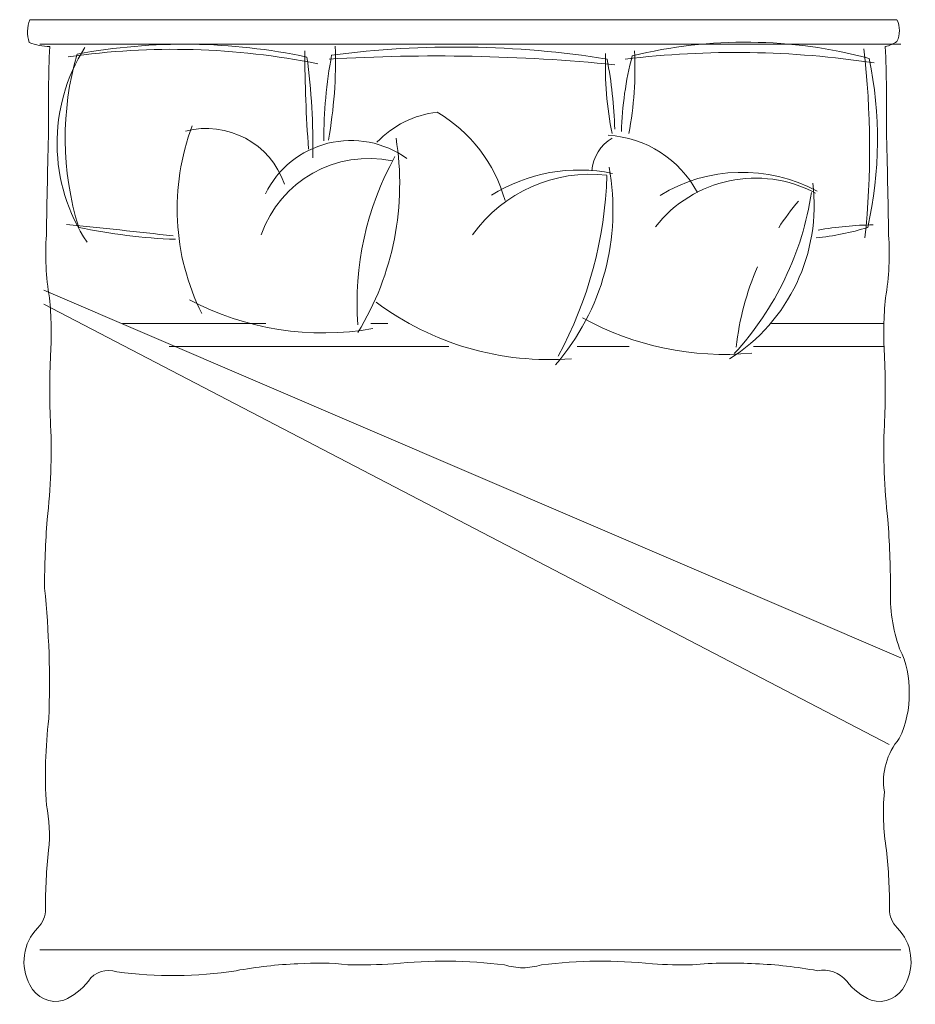
# Model space of a CAD drawing. Units: inches. Extents: x 2129 to 3258, y 1851 to 3021.
# Tile 8 of 10: x 3167.73255 to 3167.80956, y 1876.88043 to 1876.96505. Entities that reach past the tile are written whole.
import ezdxf

# ---------------------------------------------------------------- set-up
doc = ezdxf.new("R2010")
doc.units = ezdxf.units.IN
doc.layers.add('A-FURN', color=8, linetype='Continuous', lineweight=18)

# ---------------------------------------------------------------- blocks, each defined once
blk = doc.blocks.new('bed 1- king size')
at = {"color": 0}
for p, q in [((-0.9487, -0.0777), (0.9323, -0.0777)), ((-0.9394, -0.6151), (0.9323, -1.4177)), ((-0.9394, -0.6451), (0.9066, -1.6065)), ((-0.7682, -0.6873), (-0.4547, -0.6873)), ((-0.2254, -0.6873), (-0.1884, -0.6873)), ((0.6495, -0.6873), (0.8951, -0.6873)), ((-0.6659, -0.7381), (-0.0555, -0.7381)), ((0.2254, -0.7381), (0.3384, -0.7381)), ((0.6103, -0.7381), (0.8953, -0.7381)), ((-0.9487, -2.0547), (0.9323, -2.0547))]:
    blk.add_line(p, q, dxfattribs=at)
blk.add_lwpolyline([(0.898, -0.0829, 0.098699), (0.9236, -0.072, 0.222522), (0.9236, -0.0243), (-0.9705, -0.0243, 0.171621), (-0.9716, -0.0739, 0.102495), (-0.9268, -0.0829, 0.015571), (-0.9293, -0.2659, 0.00267), (-0.9341, -0.4944, 0.058958), (-0.9274, -0.6315, -0.038458), (-0.9248, -0.7552, 0.025508), (-0.9248, -0.9094, -0.039412), (-0.9326, -1.1154, 0.016498), (-0.9382, -1.2654, -0.035771), (-0.9288, -1.5502, 0.045388), (-0.9341, -1.7389, -0.080578), (-0.9295, -1.837, 0.026504), (-0.9362, -1.9656, -0.211134), (-0.9531, -2.0066, 0.329446), (-0.9701, -2.1314, 0.37589), (-0.8958, -2.1647, 0.123892), (-0.8425, -2.1233, -0.342539), (-0.78, -2.1029, 0.07104), (-0.5197, -2.1004, -0.036442), (-0.3847, -2.0853, -0.046791), (-0.2759, -2.0873, 0.023628), (-0.1759, -2.0852, -0.055897), (0.0662, -2.0877, 0.053528), (0.1067, -2.0945, 0.053528), (0.1472, -2.0877, -0.055897), (0.3893, -2.0852, 0.026973), (0.4769, -2.0873, -0.036947), (0.6147, -2.0853, -0.036442), (0.7497, -2.1004, -0.281256), (0.8137, -2.1233, -0.521995), (0.8137, -2.1233, 0.123892), (0.867, -2.1647, 0.37589), (0.9413, -2.1314, 0.329446), (0.9243, -2.0066, -0.211134), (0.9074, -1.9656, 0.026504), (0.9007, -1.837, -0.06219), (0.896, -1.7098, -0.218233), (0.9286, -1.5937, 0.123513), (0.9499, -1.4937, 0.129887), (0.9293, -1.3978, -0.095063), (0.9094, -1.2654, 0.016498), (0.9038, -1.1154, -0.039412), (0.896, -0.9094, 0.025508), (0.896, -0.7552, -0.038458), (0.8986, -0.6315, 0.058958), (0.9053, -0.4944, 0.00267), (0.9005, -0.2659, 0.015571)], format="xyb", close=True, dxfattribs=at)
for centre, radius, start, end in [((-0.5221, -0.2938), 0.3887, 147.51, 213.8336), ((-0.6323, -1.3651), 1.2872, 78.0142, 100.5125), ((-1.2482, -0.1161), 0.9455, 349.589, 2.0447), ((-0.04, -2.1818), 2.0978, 80.934, 97.4266), ((0.5931, -1.1167), 1.0433, 75.0181, 103.7392), ((-0.2311, -0.2827), 0.6619, 163.9263, 197.1409), ((-0.6569, -1.6774), 1.5884, 78.5485, 98.3029), ((2.5431, -0.0869), 2.9129, 180.1063, 184.3312), ((-1.857, -0.3037), 1.5051, 359.1536, 7.5533), ((0.7071, -0.2897), 1.0355, 169.5301, 179.934), ((-0.0818, -4.0689), 3.9654, 84.3658, 93.3969), ((1.0242, -0.1263), 0.7375, 177.8261, 191.4767), ((1.0572, -0.2894), 0.7358, 165.3434, 178.3876), ((0.5721, -2.1074), 2.0115, 81.3714, 96.917), ((-0.3946, -0.1329), 0.7459, 349.1667, 3.123), ((-1.0492, -0.3038), 1.9129, 354.0935, 6.4707), ((-0.6896, -0.2953), 0.9974, 1.8337, 10.6945), ((0.0089, -0.2863), 0.8722, 347.3175, 11.7435), ((-0.0546, -0.4435), 0.2189, 96.8992, 136.0421), ((-0.2438, -0.5051), 0.323, 15.4018, 59.7122), ((-0.1358, -0.4371), 0.5128, 159.3026, 206.5026), ((-0.5846, -0.4421), 0.1803, 18.9387, 104.6725), ((0.2786, -0.5137), 0.2374, 28.1996, 86.5061), ((-0.2688, -0.4962), 0.2082, 54.1671, 153.8421), ((-0.7873, -0.3825), 0.6248, 328.6542, 9.1977), ((0.347, -0.3604), 0.0899, 120.1134, 175.8974), ((-0.2301, -0.5756), 0.2484, 78.0413, 160.8342), ((0.4039, -0.6426), 0.6595, 151.0456, 184.1497), ((0.2545, -0.6795), 0.3178, 83.5607, 144.2853), ((0.2294, -0.7137), 0.3612, 78.4081, 122.0077), ((-0.2123, -0.4404), 0.5157, 319.1339, 10.5299), ((-0.5982, -0.336), 0.8889, 331.605, 358.1749), ((0.5856, -0.7025), 0.345, 61.6404, 121.3345), ((0.6148, -0.6485), 0.2783, 61.8876, 141.8707), ((0.3458, -0.4294), 0.3969, 302.3262, 7), ((0.0793, -0.3025), 0.6649, 317.3201, 351.4624), ((1.163, -0.8025), 0.5939, 139.9508, 146.951), ((-1.8444, -10.4721), 10.046, 83.21322, 84.54762), ((0.8799, -1.1936), 0.7214, 90.6432, 100.2707), ((-0.6059, 0.7469), 1.2515, 258.1169, 267.8849), ((0.6944, 0.0492), 0.5523, 275.447, 287.4199), ((1.163, -0.8025), 0.5939, 156.2982, 173.8539), ((-0.3293, -0.0779), 0.6301, 242.3859, 279.8951), ((0.1632, -0.137), 0.6293, 233.2201, 274.4972), ((0.5459, -0.118), 0.637, 240.9467, 275.467)]:
    blk.add_arc(centre, radius, start, end, dxfattribs=at)

msp = doc.modelspace()

# ---------------------------------------------------------------- block references
at = {"layer": 'A-FURN', "xscale": 0.0393700787401575, "yscale": 0.0393700787401575, "zscale": 0.0393700787401575}
msp.add_blockref('bed 1- king size', (3167.771622, 1876.966007), dxfattribs=at)

doc.saveas('drawing.dxf')
